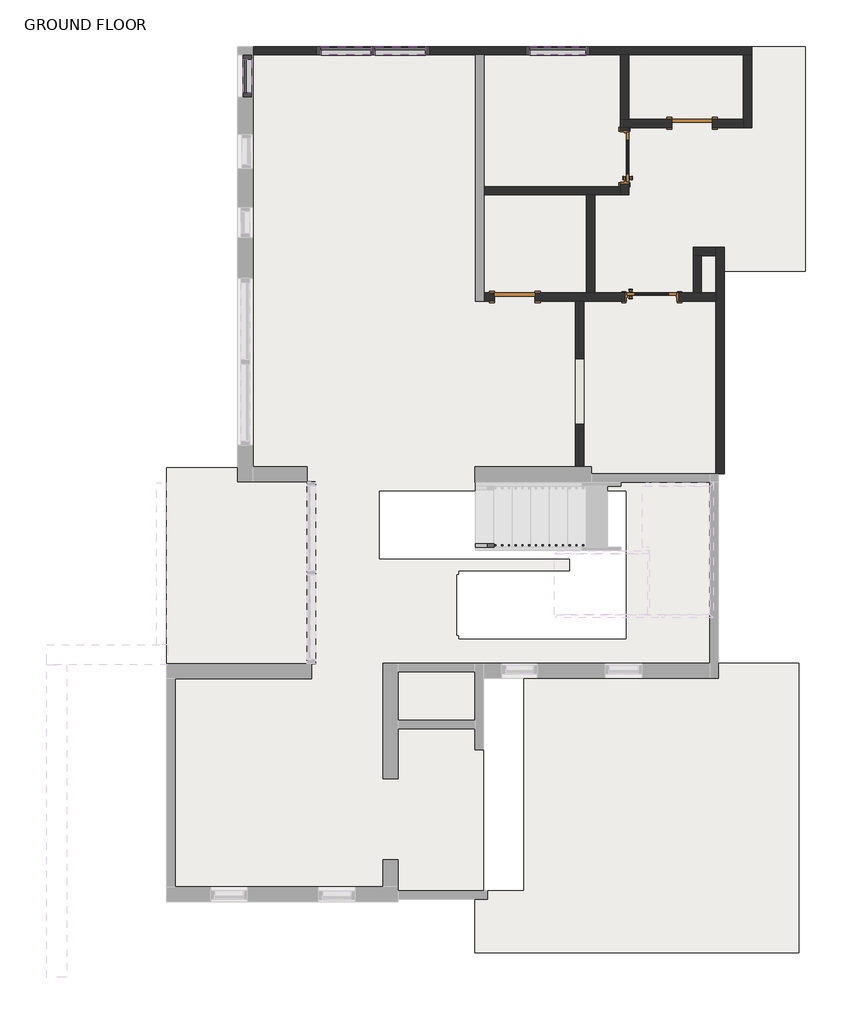
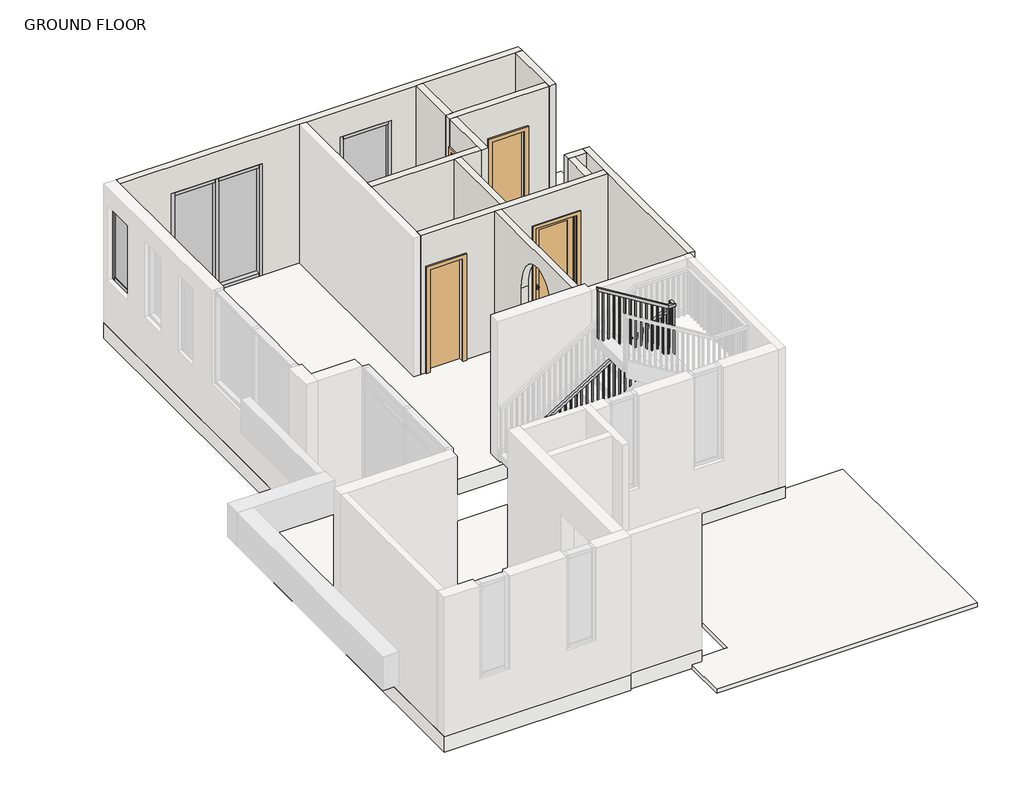
# One storey, part 2 of 3: 15 members, 12 walls, 4 doors, 4 plates, 2 slabs, 1 railing.
"""IFC4 building model written with IfcOpenShell, lengths in millimetres."""

from ifc_helpers import new_model, si_unit, point, frame, origin, origin_with_axes, place, context, project, spatial, polyline, ellipse_curve, trimmed, outline, extrude, faceted_brep, transform, mapped, element, save
from ifc_brep_helpers import plane_surface, extruded_surface, advanced_brep
from components import door_interior_single_1_panel_wood_door_3_x_7_fe7a9c6b, door_interior_single_1_panel_wood_door_3_x_7_d4f3ff50, single_flush_bathroom_2_x7_025d1c86, single_flush_bathroom_2_x7_ccebbf4d, member_de31af64, member_64030597, member_a3a7b6e3, member_71d3972c, member_e3d2676c, member_091e92f8, member_4e4be739, system_panel_glazed_14783ebf, system_panel_glazed_3c43e7a7, system_panel_glazed_fc786b5a

model = new_model("IFC4")

# Units and contexts
model_context = context("Model", 3, world=origin())
ifc_project = project(units=[si_unit("LENGTHUNIT", "METRE", prefix="MILLI")], contexts=[model_context])

# Site, building, storey
site = spatial("IfcSite", under=ifc_project)
building = spatial("IfcBuilding", under=site)
storey = spatial("IfcBuildingStorey", under=building, Name="GROUND FLOOR", Elevation=304.8)

# Doors
placement = place(None, origin())
door_interior_single_1_panel_wood_door_3_x_7_shape = door_interior_single_1_panel_wood_door_3_x_7_fe7a9c6b(model_context)
element("IfcDoor", 1, ObjectType="Door-Interior-Single-1_Panel-Wood : DOOR 3'X 7'", at=placement, inside=storey, context=model_context, shape_type="MappedRepresentation", body=[
    mapped(door_interior_single_1_panel_wood_door_3_x_7_shape, transform((-6017.3265106, -351.9048674, 304.8), x_axis=(0.0, 1.0, 0.0), y_axis=(-1.0, 0.0, 0.0), z_axis=(0.0, 0.0, 1.0))),
])
door_interior_single_1_panel_wood_door_3_x_7_2_shape = door_interior_single_1_panel_wood_door_3_x_7_d4f3ff50(model_context)
element("IfcDoor", 2, ObjectType="Door-Interior-Single-1_Panel-Wood : DOOR 3'X 7'", at=placement, inside=storey, context=model_context, shape_type="MappedRepresentation", body=[
    mapped(door_interior_single_1_panel_wood_door_3_x_7_2_shape, transform((-5610.3998675, -2456.9298674, 304.8), x_axis=(1.0, 0.0, 0.0), y_axis=(0.0, 1.0, 0.0), z_axis=(0.0, 0.0, 1.0))),
])
single_flush_bathroom_2_x7_shape = single_flush_bathroom_2_x7_025d1c86(model_context)
element("IfcDoor", 3, ObjectType="Single-Flush : BATHROOM 2' X7'", at=placement, inside=storey, context=model_context, shape_type="MappedRepresentation", body=[
    mapped(single_flush_bathroom_2_x7_shape, transform((-5004.5015106, 156.0951326, 304.8), x_axis=(1.0, 0.0, 0.0), y_axis=(0.0, 1.0, 0.0), z_axis=(0.0, 0.0, 1.0))),
])
single_flush_bathroom_2_x7_2_shape = single_flush_bathroom_2_x7_ccebbf4d(model_context)
element("IfcDoor", 4, ObjectType="Single-Flush : BATHROOM 2' X7'", at=placement, inside=storey, context=model_context, shape_type="MappedRepresentation", body=[
    mapped(single_flush_bathroom_2_x7_2_shape, transform((-7672.6911408, -2460.1048674, 304.8), x_axis=(-1.0, 0.0, 0.0), y_axis=(0.0, -1.0, 0.0), z_axis=(0.0, 0.0, 1.0))),
])

# Members
member_shape = member_de31af64(model_context)
element("IfcMember", 5, ObjectType="Rectangular Mullion : 2.5\" x 5\" rectangular", at=placement, inside=storey, context=model_context, shape_type="MappedRepresentation", body=[
    mapped(member_shape, transform((-11701.1434938, 1121.2951326, 2682.3285226), x_axis=(0.0, 0.0, 1.0), y_axis=(1.0, 0.0, 0.0), z_axis=(0.0, 1.0, 0.0))),
])
element("IfcMember", 6, ObjectType="Rectangular Mullion : 2.5\" x 5\" rectangular", at=placement, inside=storey, context=model_context, shape_type="MappedRepresentation", body=[
    mapped(member_shape, transform((-11701.1434938, 614.3802108, 1219.2), x_axis=(0.0, 0.0, -1.0), y_axis=(1.0, 0.0, 0.0), z_axis=(0.0, -1.0, 0.0))),
])
member_2_shape = member_64030597(model_context)
element("IfcMember", 7, ObjectType="Rectangular Mullion : 2.5\" x 5\" rectangular", at=placement, inside=storey, context=model_context, shape_type="MappedRepresentation", body=[
    mapped(member_2_shape, transform((-11701.1434938, 1184.7951326, 1219.2), x_axis=(0.0, 1.0, 0.0), y_axis=(1.0, 0.0, 0.0), z_axis=(0.0, 0.0, -1.0))),
])
element("IfcMember", 8, ObjectType="Rectangular Mullion : 2.5\" x 5\" rectangular", at=placement, inside=storey, context=model_context, shape_type="MappedRepresentation", body=[
    mapped(member_2_shape, transform((-11701.1434938, 550.8802108, 2682.3285226), x_axis=(0.0, -1.0, 0.0), y_axis=(1.0, 0.0, 0.0), z_axis=(0.0, 0.0, 1.0))),
])
member_3_shape = member_a3a7b6e3(model_context)
element("IfcMember", 9, ObjectType="Rectangular Mullion : 2.5\" x 5\" rectangular", at=placement, inside=storey, context=model_context, shape_type="MappedRepresentation", body=[
    mapped(member_3_shape, transform((-9021.4434938, 1248.2951326, 2512.8093941), x_axis=(0.0, 0.0, 1.0), y_axis=(0.0, -1.0, 0.0), z_axis=(1.0, 0.0, 0.0))),
])
element("IfcMember", 10, ObjectType="Rectangular Mullion : 2.5\" x 5\" rectangular", at=placement, inside=storey, context=model_context, shape_type="MappedRepresentation", body=[
    mapped(member_3_shape, transform((-9840.5934938, 1248.2951326, 2512.8093941), x_axis=(0.0, 0.0, 1.0), y_axis=(0.0, -1.0, 0.0), z_axis=(1.0, 0.0, 0.0))),
])
element("IfcMember", 11, ObjectType="Rectangular Mullion : 2.5\" x 5\" rectangular", at=placement, inside=storey, context=model_context, shape_type="MappedRepresentation", body=[
    mapped(member_3_shape, transform((-10596.2434938, 1248.2951326, 304.8), x_axis=(0.0, 0.0, -1.0), y_axis=(0.0, -1.0, 0.0), z_axis=(-1.0, 0.0, 0.0))),
])
element("IfcMember", 12, ObjectType="Rectangular Mullion : 2.5\" x 5\" rectangular", at=placement, inside=storey, context=model_context, shape_type="MappedRepresentation", body=[
    mapped(member_3_shape, transform((-9777.0934938, 1248.2951326, 304.8), x_axis=(0.0, 0.0, -1.0), y_axis=(0.0, -1.0, 0.0), z_axis=(-1.0, 0.0, 0.0))),
])
member_4_shape = member_71d3972c(model_context)
element("IfcMember", 13, ObjectType="Rectangular Mullion : 2.5\" x 5\" rectangular", at=placement, inside=storey, context=model_context, shape_type="MappedRepresentation", body=[
    mapped(member_4_shape, transform((-9808.8434938, 1248.2951326, 304.8), x_axis=(1.0, 0.0, 0.0), y_axis=(0.0, -1.0, 0.0), z_axis=(0.0, 0.0, -1.0))),
])
member_5_shape = member_e3d2676c(model_context)
element("IfcMember", 14, ObjectType="Rectangular Mullion : 2.5\" x 5\" rectangular", at=placement, inside=storey, context=model_context, shape_type="MappedRepresentation", body=[
    mapped(member_5_shape, transform((-8957.9434938, 1248.2951326, 304.8), x_axis=(1.0, 0.0, 0.0), y_axis=(0.0, -1.0, 0.0), z_axis=(0.0, 0.0, -1.0))),
])
element("IfcMember", 15, ObjectType="Rectangular Mullion : 2.5\" x 5\" rectangular", at=placement, inside=storey, context=model_context, shape_type="MappedRepresentation", body=[
    mapped(member_5_shape, transform((-10659.7434938, 1248.2951326, 2512.8093941), x_axis=(-1.0, 0.0, 0.0), y_axis=(0.0, -1.0, 0.0), z_axis=(0.0, 0.0, 1.0))),
])
member_6_shape = member_091e92f8(model_context)
element("IfcMember", 16, ObjectType="Rectangular Mullion : 2.5\" x 5\" rectangular", at=placement, inside=storey, context=model_context, shape_type="MappedRepresentation", body=[
    mapped(member_6_shape, transform((-6603.3899211, 1248.2951326, 2525.2042846), x_axis=(0.0, 0.0, 1.0), y_axis=(0.0, -1.0, 0.0), z_axis=(1.0, 0.0, 0.0))),
])
element("IfcMember", 17, ObjectType="Rectangular Mullion : 2.5\" x 5\" rectangular", at=placement, inside=storey, context=model_context, shape_type="MappedRepresentation", body=[
    mapped(member_6_shape, transform((-7447.9399211, 1248.2951326, 304.8), x_axis=(0.0, 0.0, -1.0), y_axis=(0.0, -1.0, 0.0), z_axis=(-1.0, 0.0, 0.0))),
])
member_7_shape = member_4e4be739(model_context)
element("IfcMember", 18, ObjectType="Rectangular Mullion : 2.5\" x 5\" rectangular", at=placement, inside=storey, context=model_context, shape_type="MappedRepresentation", body=[
    mapped(member_7_shape, transform((-6539.8899211, 1248.2951326, 304.8), x_axis=(1.0, 0.0, 0.0), y_axis=(0.0, -1.0, 0.0), z_axis=(0.0, 0.0, -1.0))),
])
element("IfcMember", 19, ObjectType="Rectangular Mullion : 2.5\" x 5\" rectangular", at=placement, inside=storey, context=model_context, shape_type="MappedRepresentation", body=[
    mapped(member_7_shape, transform((-7511.4399211, 1248.2951326, 2525.2042846), x_axis=(-1.0, 0.0, 0.0), y_axis=(0.0, -1.0, 0.0), z_axis=(0.0, 0.0, 1.0))),
])

# Plates
system_panel_glazed_shape = system_panel_glazed_14783ebf(model_context)
element("IfcPlate", 20, ObjectType="System Panel : Glazed", at=placement, inside=storey, context=model_context, shape_type="MappedRepresentation", body=[
    mapped(system_panel_glazed_shape, transform((-11701.1434938, 867.8376717, 1282.7), x_axis=(0.0, 1.0, 0.0), y_axis=(-1.0, 0.0, 0.0), z_axis=(0.0, 0.0, 1.0))),
])
system_panel_glazed_2_shape = system_panel_glazed_3c43e7a7(model_context)
element("IfcPlate", 21, ObjectType="System Panel : Glazed", at=placement, inside=storey, context=model_context, shape_type="MappedRepresentation", body=[
    mapped(system_panel_glazed_2_shape, transform((-10218.4184938, 1248.2951326, 368.3), x_axis=(1.0, 0.0, 0.0), y_axis=(0.0, 1.0, 0.0), z_axis=(0.0, 0.0, 1.0))),
])
element("IfcPlate", 22, ObjectType="System Panel : Glazed", at=placement, inside=storey, context=model_context, shape_type="MappedRepresentation", body=[
    mapped(system_panel_glazed_2_shape, transform((-9399.2684938, 1248.2951326, 368.3), x_axis=(1.0, 0.0, 0.0), y_axis=(0.0, 1.0, 0.0), z_axis=(0.0, 0.0, 1.0))),
])
system_panel_glazed_3_shape = system_panel_glazed_fc786b5a(model_context)
element("IfcPlate", 23, ObjectType="System Panel : Glazed", at=placement, inside=storey, context=model_context, shape_type="MappedRepresentation", body=[
    mapped(system_panel_glazed_3_shape, transform((-7025.6649211, 1248.2951326, 368.3), x_axis=(1.0, 0.0, 0.0), y_axis=(0.0, 1.0, 0.0), z_axis=(0.0, 0.0, 1.0))),
])

# Railing
element("IfcRailing", 24, ObjectType="Handrail - Rectangular", at=placement, inside=storey, context=model_context, shape_type="SolidModel", body=[
    faceted_brep([(-8269.5911408, -6173.9337491, 1390.65), (-8269.5911408, -6173.9337491, 1331.0481634), (-8269.5911408, -6224.7337491, 1331.0481634), (-8269.5911408, -6224.7337491, 1390.65), (-5754.9911408, -6173.9337491, 2933.7), (-5740.6474071, -6173.9337491, 2882.9), (-5740.6474071, -6224.7337491, 2882.9), (-5754.9911408, -6224.7337491, 2933.7), (-5596.7260609, -6173.9337491, 2933.7), (-5596.7260609, -6173.9337491, 2882.9), (-5647.5260609, -6224.7337491, 2882.9), (-5647.5260609, -6224.7337491, 2933.7), (-5596.7260609, -6251.7310793, 2933.7), (-5596.7260609, -6302.5310793, 2882.9), (-5647.5260609, -6302.5310793, 2882.9), (-5647.5260609, -6251.7310793, 2933.7), (-5596.7260609, -6251.7310793, 3151.9090909), (-5596.7260609, -6302.5310793, 3101.1090909), (-5647.5260609, -6302.5310793, 3101.1090909), (-5647.5260609, -6251.7310793, 3151.9090909), (-5596.7260609, -6378.7310793, 3151.9090909), (-5596.7260609, -6378.7310793, 3101.1090909), (-5647.5260609, -6327.9310793, 3101.1090909), (-5647.5260609, -6327.9310793, 3151.9090909), (-5723.7260609, -6378.7310793, 3151.9090909), (-5738.0697946, -6378.7310793, 3101.1090909), (-5738.0697946, -6327.9310793, 3101.1090909), (-5723.7260609, -6327.9310793, 3151.9090909), (-7044.5260609, -6378.7310793, 3962.4), (-7044.5260609, -6327.9310793, 3962.4), (-7044.5260609, -6327.9310793, 3902.7981634), (-7044.5260609, -6378.7310793, 3902.7981634)], [[[0, 1, 2, 3]], [[1, 0, 4, 5]], [[2, 1, 5, 6]], [[3, 2, 6, 7]], [[0, 3, 7, 4]], [[5, 4, 8, 9]], [[6, 5, 9, 10]], [[7, 6, 10, 11]], [[4, 7, 11, 8]], [[9, 8, 12, 13]], [[10, 9, 13, 14]], [[11, 10, 14, 15]], [[8, 11, 15, 12]], [[13, 12, 16, 17]], [[14, 13, 17, 18]], [[15, 14, 18, 19]], [[12, 15, 19, 16]], [[17, 16, 20, 21]], [[18, 17, 21, 22]], [[19, 18, 22, 23]], [[16, 19, 23, 20]], [[21, 20, 24, 25]], [[22, 21, 25, 26]], [[23, 22, 26, 27]], [[20, 23, 27, 24]], [[28, 29, 30, 31]], [[25, 24, 28, 31]], [[26, 25, 31, 30]], [[27, 26, 30, 29]], [[24, 27, 29, 28]]]),
    extrude(outline(polyline([(3834.6078225, -6933.4010609), (3846.2975952, -6952.4510609), (2876.55, -6952.4510609), (2876.55, -6933.4010609), (3834.6078225, -6933.4010609)])), frame((0.0, -6362.8560793, 0.0), z_axis=(0.0, 1.0, 0.0), x_axis=(0.0, 0.0, 1.0)), (0.0, 0.0, 1.0), 19.05),
    extrude(outline(polyline([(3772.2623679, -6831.8010609), (3783.9521407, -6850.8510609), (2876.55, -6850.8510609), (2876.55, -6831.8010609), (3772.2623679, -6831.8010609)])), frame((0.0, -6362.8560793, 0.0), z_axis=(0.0, 1.0, 0.0), x_axis=(0.0, 0.0, 1.0)), (0.0, 0.0, 1.0), 19.05),
    extrude(outline(polyline([(3709.9169134, -6730.2010609), (3721.6066861, -6749.2510609), (2705.1, -6749.2510609), (2705.1, -6730.2010609), (3709.9169134, -6730.2010609)])), frame((0.0, -6362.8560793, 0.0), z_axis=(0.0, 1.0, 0.0), x_axis=(0.0, 0.0, 1.0)), (0.0, 0.0, 1.0), 19.05),
    extrude(outline(polyline([(3647.5714589, -6628.6010609), (3659.2612316, -6647.6510609), (2705.1, -6647.6510609), (2705.1, -6628.6010609), (3647.5714589, -6628.6010609)])), frame((0.0, -6362.8560793, 0.0), z_axis=(0.0, 1.0, 0.0), x_axis=(0.0, 0.0, 1.0)), (0.0, 0.0, 1.0), 19.05),
    extrude(outline(polyline([(3585.2260043, -6527.0010609), (3596.915777, -6546.0510609), (2705.1, -6546.0510609), (2705.1, -6527.0010609), (3585.2260043, -6527.0010609)])), frame((0.0, -6362.8560793, 0.0), z_axis=(0.0, 1.0, 0.0), x_axis=(0.0, 0.0, 1.0)), (0.0, 0.0, 1.0), 19.05),
    extrude(outline(polyline([(3522.8805498, -6425.4010609), (3534.5703225, -6444.4510609), (2533.65, -6444.4510609), (2533.65, -6425.4010609), (3522.8805498, -6425.4010609)])), frame((0.0, -6362.8560793, 0.0), z_axis=(0.0, 1.0, 0.0), x_axis=(0.0, 0.0, 1.0)), (0.0, 0.0, 1.0), 19.05),
    extrude(outline(polyline([(3460.5350952, -6323.8010609), (3472.2248679, -6342.8510609), (2533.65, -6342.8510609), (2533.65, -6323.8010609), (3460.5350952, -6323.8010609)])), frame((0.0, -6362.8560793, 0.0), z_axis=(0.0, 1.0, 0.0), x_axis=(0.0, 0.0, 1.0)), (0.0, 0.0, 1.0), 19.05),
    extrude(outline(polyline([(3398.1896407, -6222.2010609), (3409.8794134, -6241.2510609), (2533.65, -6241.2510609), (2533.65, -6222.2010609), (3398.1896407, -6222.2010609)])), frame((0.0, -6362.8560793, 0.0), z_axis=(0.0, 1.0, 0.0), x_axis=(0.0, 0.0, 1.0)), (0.0, 0.0, 1.0), 19.05),
    extrude(outline(polyline([(3335.8441861, -6120.6010609), (3347.5339589, -6139.6510609), (2362.2, -6139.6510609), (2362.2, -6120.6010609), (3335.8441861, -6120.6010609)])), frame((0.0, -6362.8560793, 0.0), z_axis=(0.0, 1.0, 0.0), x_axis=(0.0, 0.0, 1.0)), (0.0, 0.0, 1.0), 19.05),
    extrude(outline(polyline([(3273.4987316, -6019.0010609), (3285.1885043, -6038.0510609), (2362.2, -6038.0510609), (2362.2, -6019.0010609), (3273.4987316, -6019.0010609)])), frame((0.0, -6362.8560793, 0.0), z_axis=(0.0, 1.0, 0.0), x_axis=(0.0, 0.0, 1.0)), (0.0, 0.0, 1.0), 19.05),
    extrude(outline(polyline([(3211.153277, -5917.4010609), (3222.8430498, -5936.4510609), (2362.2, -5936.4510609), (2362.2, -5917.4010609), (3211.153277, -5917.4010609)])), frame((0.0, -6362.8560793, 0.0), z_axis=(0.0, 1.0, 0.0), x_axis=(0.0, 0.0, 1.0)), (0.0, 0.0, 1.0), 19.05),
    extrude(outline(polyline([(3148.8078225, -5815.8010609), (3160.4975952, -5834.8510609), (2190.75, -5834.8510609), (2190.75, -5815.8010609), (3148.8078225, -5815.8010609)])), frame((0.0, -6362.8560793, 0.0), z_axis=(0.0, 1.0, 0.0), x_axis=(0.0, 0.0, 1.0)), (0.0, 0.0, 1.0), 19.05),
    extrude(outline(polyline([(3086.4623679, -5714.2010609), (3098.1521407, -5733.2510609), (2190.75, -5733.2510609), (2190.75, -5714.2010609), (3086.4623679, -5714.2010609)])), frame((0.0, -6362.8560793, 0.0), z_axis=(0.0, 1.0, 0.0), x_axis=(0.0, 0.0, 1.0)), (0.0, 0.0, 1.0), 19.05),
    extrude(outline(polyline([(-5631.6510609, -6291.4087491), (-5612.6010609, -6291.4087491), (-5612.6010609, -6310.4587491), (-5631.6510609, -6310.4587491), (-5631.6510609, -6291.4087491)])), frame((0.0, 0.0, 2019.3), z_axis=(0.0, 0.0, 1.0), x_axis=(1.0, 0.0, 0.0)), (0.0, 0.0, 1.0), 1081.8090909),
    extrude(outline(polyline([(-5662.9161408, -6208.8587491), (-5662.9161408, -6189.8087491), (-5643.8661408, -6189.8087491), (-5643.8661408, -6208.8587491), (-5662.9161408, -6208.8587491)])), frame((0.0, 0.0, 2019.3), z_axis=(0.0, 0.0, 1.0), x_axis=(1.0, 0.0, 0.0)), (0.0, 0.0, 1.0), 863.6),
    extrude(outline(polyline([(2833.1839589, -5821.6661408), (2821.4941861, -5840.7161408), (1847.85, -5840.7161408), (1847.85, -5821.6661408), (2833.1839589, -5821.6661408)])), frame((0.0, -6208.8587491, 0.0), z_axis=(0.0, 1.0, 0.0), x_axis=(0.0, 0.0, 1.0)), (0.0, 0.0, 1.0), 19.05),
    extrude(outline(polyline([(2770.8385043, -5923.2661408), (2759.1487316, -5942.3161408), (1847.85, -5942.3161408), (1847.85, -5923.2661408), (2770.8385043, -5923.2661408)])), frame((0.0, -6208.8587491, 0.0), z_axis=(0.0, 1.0, 0.0), x_axis=(0.0, 0.0, 1.0)), (0.0, 0.0, 1.0), 19.05),
    extrude(outline(polyline([(2708.4930498, -6024.8661408), (2696.803277, -6043.9161408), (1847.85, -6043.9161408), (1847.85, -6024.8661408), (2708.4930498, -6024.8661408)])), frame((0.0, -6208.8587491, 0.0), z_axis=(0.0, 1.0, 0.0), x_axis=(0.0, 0.0, 1.0)), (0.0, 0.0, 1.0), 19.05),
    extrude(outline(polyline([(2646.1475952, -6126.4661408), (2634.4578225, -6145.5161408), (1676.4, -6145.5161408), (1676.4, -6126.4661408), (2646.1475952, -6126.4661408)])), frame((0.0, -6208.8587491, 0.0), z_axis=(0.0, 1.0, 0.0), x_axis=(0.0, 0.0, 1.0)), (0.0, 0.0, 1.0), 19.05),
    extrude(outline(polyline([(2583.8021407, -6228.0661408), (2572.1123679, -6247.1161408), (1676.4, -6247.1161408), (1676.4, -6228.0661408), (2583.8021407, -6228.0661408)])), frame((0.0, -6208.8587491, 0.0), z_axis=(0.0, 1.0, 0.0), x_axis=(0.0, 0.0, 1.0)), (0.0, 0.0, 1.0), 19.05),
    extrude(outline(polyline([(2521.4566861, -6329.6661408), (2509.7669134, -6348.7161408), (1504.95, -6348.7161408), (1504.95, -6329.6661408), (2521.4566861, -6329.6661408)])), frame((0.0, -6208.8587491, 0.0), z_axis=(0.0, 1.0, 0.0), x_axis=(0.0, 0.0, 1.0)), (0.0, 0.0, 1.0), 19.05),
    extrude(outline(polyline([(2459.1112316, -6431.2661408), (2447.4214589, -6450.3161408), (1504.95, -6450.3161408), (1504.95, -6431.2661408), (2459.1112316, -6431.2661408)])), frame((0.0, -6208.8587491, 0.0), z_axis=(0.0, 1.0, 0.0), x_axis=(0.0, 0.0, 1.0)), (0.0, 0.0, 1.0), 19.05),
    extrude(outline(polyline([(2396.765777, -6532.8661408), (2385.0760043, -6551.9161408), (1504.95, -6551.9161408), (1504.95, -6532.8661408), (2396.765777, -6532.8661408)])), frame((0.0, -6208.8587491, 0.0), z_axis=(0.0, 1.0, 0.0), x_axis=(0.0, 0.0, 1.0)), (0.0, 0.0, 1.0), 19.05),
    extrude(outline(polyline([(2334.4203225, -6634.4661408), (2322.7305498, -6653.5161408), (1333.5, -6653.5161408), (1333.5, -6634.4661408), (2334.4203225, -6634.4661408)])), frame((0.0, -6208.8587491, 0.0), z_axis=(0.0, 1.0, 0.0), x_axis=(0.0, 0.0, 1.0)), (0.0, 0.0, 1.0), 19.05),
    extrude(outline(polyline([(2272.0748679, -6736.0661408), (2260.3850952, -6755.1161408), (1333.5, -6755.1161408), (1333.5, -6736.0661408), (2272.0748679, -6736.0661408)])), frame((0.0, -6208.8587491, 0.0), z_axis=(0.0, 1.0, 0.0), x_axis=(0.0, 0.0, 1.0)), (0.0, 0.0, 1.0), 19.05),
    extrude(outline(polyline([(2209.7294134, -6837.6661408), (2198.0396407, -6856.7161408), (1333.5, -6856.7161408), (1333.5, -6837.6661408), (2209.7294134, -6837.6661408)])), frame((0.0, -6208.8587491, 0.0), z_axis=(0.0, 1.0, 0.0), x_axis=(0.0, 0.0, 1.0)), (0.0, 0.0, 1.0), 19.05),
    extrude(outline(polyline([(2147.3839589, -6939.2661408), (2135.6941861, -6958.3161408), (1162.05, -6958.3161408), (1162.05, -6939.2661408), (2147.3839589, -6939.2661408)])), frame((0.0, -6208.8587491, 0.0), z_axis=(0.0, 1.0, 0.0), x_axis=(0.0, 0.0, 1.0)), (0.0, 0.0, 1.0), 19.05),
    extrude(outline(polyline([(2085.0385043, -7040.8661408), (2073.3487316, -7059.9161408), (1162.05, -7059.9161408), (1162.05, -7040.8661408), (2085.0385043, -7040.8661408)])), frame((0.0, -6208.8587491, 0.0), z_axis=(0.0, 1.0, 0.0), x_axis=(0.0, 0.0, 1.0)), (0.0, 0.0, 1.0), 19.05),
    extrude(outline(polyline([(2022.6930498, -7142.4661408), (2011.003277, -7161.5161408), (1162.05, -7161.5161408), (1162.05, -7142.4661408), (2022.6930498, -7142.4661408)])), frame((0.0, -6208.8587491, 0.0), z_axis=(0.0, 1.0, 0.0), x_axis=(0.0, 0.0, 1.0)), (0.0, 0.0, 1.0), 19.05),
    extrude(outline(polyline([(1960.3475952, -7244.0661408), (1948.6578225, -7263.1161408), (990.6, -7263.1161408), (990.6, -7244.0661408), (1960.3475952, -7244.0661408)])), frame((0.0, -6208.8587491, 0.0), z_axis=(0.0, 1.0, 0.0), x_axis=(0.0, 0.0, 1.0)), (0.0, 0.0, 1.0), 19.05),
    extrude(outline(polyline([(1898.0021407, -7345.6661408), (1886.3123679, -7364.7161408), (990.6, -7364.7161408), (990.6, -7345.6661408), (1898.0021407, -7345.6661408)])), frame((0.0, -6208.8587491, 0.0), z_axis=(0.0, 1.0, 0.0), x_axis=(0.0, 0.0, 1.0)), (0.0, 0.0, 1.0), 19.05),
    extrude(outline(polyline([(1835.6566861, -7447.2661408), (1823.9669134, -7466.3161408), (819.15, -7466.3161408), (819.15, -7447.2661408), (1835.6566861, -7447.2661408)])), frame((0.0, -6208.8587491, 0.0), z_axis=(0.0, 1.0, 0.0), x_axis=(0.0, 0.0, 1.0)), (0.0, 0.0, 1.0), 19.05),
    extrude(outline(polyline([(1773.3112316, -7548.8661408), (1761.6214589, -7567.9161408), (819.15, -7567.9161408), (819.15, -7548.8661408), (1773.3112316, -7548.8661408)])), frame((0.0, -6208.8587491, 0.0), z_axis=(0.0, 1.0, 0.0), x_axis=(0.0, 0.0, 1.0)), (0.0, 0.0, 1.0), 19.05),
    extrude(outline(polyline([(1710.965777, -7650.4661408), (1699.2760043, -7669.5161408), (819.15, -7669.5161408), (819.15, -7650.4661408), (1710.965777, -7650.4661408)])), frame((0.0, -6208.8587491, 0.0), z_axis=(0.0, 1.0, 0.0), x_axis=(0.0, 0.0, 1.0)), (0.0, 0.0, 1.0), 19.05),
    extrude(outline(polyline([(1648.6203225, -7752.0661408), (1636.9305498, -7771.1161408), (647.7, -7771.1161408), (647.7, -7752.0661408), (1648.6203225, -7752.0661408)])), frame((0.0, -6208.8587491, 0.0), z_axis=(0.0, 1.0, 0.0), x_axis=(0.0, 0.0, 1.0)), (0.0, 0.0, 1.0), 19.05),
    extrude(outline(polyline([(1586.2748679, -7853.6661408), (1574.5850952, -7872.7161408), (647.7, -7872.7161408), (647.7, -7853.6661408), (1586.2748679, -7853.6661408)])), frame((0.0, -6208.8587491, 0.0), z_axis=(0.0, 1.0, 0.0), x_axis=(0.0, 0.0, 1.0)), (0.0, 0.0, 1.0), 19.05),
    extrude(outline(polyline([(1523.9294134, -7955.2661408), (1512.2396407, -7974.3161408), (647.7, -7974.3161408), (647.7, -7955.2661408), (1523.9294134, -7955.2661408)])), frame((0.0, -6208.8587491, 0.0), z_axis=(0.0, 1.0, 0.0), x_axis=(0.0, 0.0, 1.0)), (0.0, 0.0, 1.0), 19.05),
    extrude(outline(polyline([(1461.5839589, -8056.8661408), (1449.8941861, -8075.9161408), (476.25, -8075.9161408), (476.25, -8056.8661408), (1461.5839589, -8056.8661408)])), frame((0.0, -6208.8587491, 0.0), z_axis=(0.0, 1.0, 0.0), x_axis=(0.0, 0.0, 1.0)), (0.0, 0.0, 1.0), 19.05),
    extrude(outline(polyline([(1399.2385043, -8158.4661408), (1387.5487316, -8177.5161408), (476.25, -8177.5161408), (476.25, -8158.4661408), (1399.2385043, -8158.4661408)])), frame((0.0, -6208.8587491, 0.0), z_axis=(0.0, 1.0, 0.0), x_axis=(0.0, 0.0, 1.0)), (0.0, 0.0, 1.0), 19.05),
    extrude(outline(polyline([(-5631.6510609, -6343.8060793), (-5612.6010609, -6343.8060793), (-5612.6010609, -6362.8560793), (-5631.6510609, -6362.8560793), (-5631.6510609, -6343.8060793)])), frame((0.0, 0.0, 2019.3), z_axis=(0.0, 0.0, 1.0), x_axis=(1.0, 0.0, 0.0)), (0.0, 0.0, 1.0), 1081.8090909),
    extrude(outline(polyline([(-5631.6510609, -6208.8587491), (-5631.6510609, -6189.8087491), (-5612.6010609, -6189.8087491), (-5612.6010609, -6208.8587491), (-5631.6510609, -6208.8587491)])), frame((0.0, 0.0, 2019.3), z_axis=(0.0, 0.0, 1.0), x_axis=(1.0, 0.0, 0.0)), (0.0, 0.0, 1.0), 863.6),
    extrude(outline(polyline([(2879.9430498, -5745.4661408), (2868.253277, -5764.5161408), (2019.3, -5764.5161408), (2019.3, -5745.4661408), (2879.9430498, -5745.4661408)])), frame((0.0, -6208.8587491, 0.0), z_axis=(0.0, 1.0, 0.0), x_axis=(0.0, 0.0, 1.0)), (0.0, 0.0, 1.0), 19.05),
    extrude(outline(polyline([(3891.1083907, -7025.4760609), (3902.7981634, -7044.5260609), (2876.55, -7044.5260609), (2876.55, -7025.4760609), (3891.1083907, -7025.4760609)])), frame((0.0, -6362.8560793, 0.0), z_axis=(0.0, 1.0, 0.0), x_axis=(0.0, 0.0, 1.0)), (0.0, 0.0, 1.0), 19.05),
    extrude(outline(polyline([(1342.7379361, -8250.5411408), (1331.0481634, -8269.5911408), (476.25, -8269.5911408), (476.25, -8250.5411408), (1342.7379361, -8250.5411408)])), frame((0.0, -6208.8587491, 0.0), z_axis=(0.0, 1.0, 0.0), x_axis=(0.0, 0.0, 1.0)), (0.0, 0.0, 1.0), 19.05),
])

# Slabs
element("IfcSlab", 25, ObjectType="MARBLE FLOORING 1'", at=placement, inside=storey, context=model_context, shape_type="SweptSolid", body=[
    extrude(outline(polyline([(-8087.622653, -11530.1453012), (-9433.822653, -11530.1453012), (-9433.822653, -11568.2453012), (-12920.5906521, -11568.2453012), (-12920.5906521, -5027.4864969), (-11849.8015106, -5027.4864969), (-11849.8015106, 1311.7951326), (-3297.4727979, 1311.7951326), (-3297.4727979, -2071.8337491), (-4516.6727979, -2071.8337491), (-4516.6727979, -5119.8337491), (-4605.5727979, -5119.8337491), (-4605.5727979, -8203.7830995), (-8147.3960918, -8203.7830995), (-8147.3960918, -11403.1453012), (-8087.622653, -11403.1453012), (-8087.622653, -11530.1453012)]), holes=[polyline([(-8549.4760609, -7553.4810793), (-8517.7260609, -7553.4810793), (-8517.7260609, -7604.2810793), (-6003.1260609, -7604.2810793), (-6003.1260609, -5382.5504041), (-9709.3703437, -5382.5504041), (-9709.3703437, -6398.5504041), (-6841.3260609, -6398.5504041), (-6841.3260609, -6588.2810793), (-8517.7260609, -6588.2810793), (-8517.7260609, -6639.0810793), (-8549.4760609, -6639.0810793), (-8549.4760609, -7553.4810793)])]), origin_with_axes(), (0.0, 0.0, 1.0), 304.8),
])
element("IfcSlab", 26, ObjectType="VERANDA FLOORING 3\"", at=placement, inside=storey, context=model_context, shape_type="SweptSolid", body=[
    extrude(outline(polyline([(-3395.0260735, -7975.1830995), (-3395.0260735, -12330.4921987), (-8271.8260735, -12330.4921987), (-8271.8260735, -11530.1453012), (-8087.622653, -11530.1453012), (-8087.622653, -11403.1453012), (-7537.7960918, -11403.1453012), (-7537.7960918, -8203.7830995), (-4605.5727979, -8203.7830995), (-4605.5727979, -7975.1830995), (-3395.0260735, -7975.1830995)])), origin_with_axes(), (0.0, 0.0, 1.0), 76.2),
])

# Walls
element("IfcWall", 27, ObjectType="INTERIOR WALL PAINT 5\"", at=placement, inside=storey, context=model_context, shape_type="Brep", body=[
    faceted_brep([(-4102.8015106, 1184.7951326, 3048.0), (-4229.8015106, 1184.7951326, 3048.0), (-5957.0015106, 1184.7951326, 3048.0), (-6084.0015106, 1184.7951326, 3048.0), (-8142.5911408, 1184.7951326, 3048.0), (-8269.5911408, 1184.7951326, 3048.0), (-11621.2015106, 1184.7951326, 3048.0), (-11621.2015106, 1184.7951326, 2682.3285226), (-11621.2015106, 1184.7951326, 1219.2), (-11621.2015106, 1184.7951326, 304.8), (-10659.7434938, 1184.7951326, 304.8), (-10659.7434938, 1184.7951326, 2512.8093941), (-8957.9434938, 1184.7951326, 2512.8093941), (-8957.9434938, 1184.7951326, 304.8), (-8269.5911408, 1184.7951326, 304.8), (-8142.5911408, 1184.7951326, 304.8), (-7511.4399211, 1184.7951326, 304.8), (-7511.4399211, 1184.7951326, 2525.2042846), (-6539.8899211, 1184.7951326, 2525.2042846), (-6539.8899211, 1184.7951326, 304.8), (-6084.0015106, 1184.7951326, 304.8), (-5957.0015106, 1184.7951326, 304.8), (-4229.8015106, 1184.7951326, 304.8), (-4102.8015106, 1184.7951326, 304.8), (-11621.2015106, 1311.7951326, 3048.0), (-4102.8015106, 1311.7951326, 3048.0), (-4102.8015106, 1311.7951326, 304.8), (-6539.8899211, 1311.7951326, 304.8), (-6539.8899211, 1311.7951326, 2525.2042846), (-7511.4399211, 1311.7951326, 2525.2042846), (-7511.4399211, 1311.7951326, 304.8), (-8957.9434938, 1311.7951326, 304.8), (-8957.9434938, 1311.7951326, 2512.8093941), (-10659.7434938, 1311.7951326, 2512.8093941), (-10659.7434938, 1311.7951326, 304.8), (-11621.2015106, 1311.7951326, 304.8)], [[[0, 1, 2, 3, 4, 5, 6, 7, 8, 9, 10, 11, 12, 13, 14, 15, 16, 17, 18, 19, 20, 21, 22, 23]], [[24, 25, 26, 27, 28, 29, 30, 31, 32, 33, 34, 35]], [[9, 35, 34, 10]], [[26, 23, 22, 21, 20, 19, 27]], [[13, 31, 30, 16, 15, 14]], [[6, 5, 4, 3, 2, 1, 0, 25, 24]], [[9, 8, 7, 6, 24, 35]], [[0, 23, 26, 25]], [[33, 11, 10, 34]], [[11, 33, 32, 12]], [[12, 32, 31, 13]], [[29, 17, 16, 30]], [[17, 29, 28, 18]], [[18, 28, 27, 19]]]),
])
element("IfcWall", 28, ObjectType="INTERIOR WALL PAINT 5\"", at=placement, inside=storey, context=model_context, shape_type="Brep", body=[
    faceted_brep([(-4229.8015106, 1184.7951326, 304.8), (-4229.8015106, 219.5951326, 304.8), (-4229.8015106, 92.5951326, 304.8), (-4229.8015106, 92.5951326, 3048.0), (-4229.8015106, 219.5951326, 3048.0), (-4229.8015106, 1184.7951326, 3048.0), (-4102.8015106, 1184.7951326, 304.8), (-4102.8015106, 1184.7951326, 3048.0), (-4102.8015106, 92.5951326, 3048.0), (-4102.8015106, 92.5951326, 304.8)], [[[0, 1, 2, 3, 4, 5]], [[6, 7, 8, 9]], [[2, 1, 0, 6, 9]], [[5, 4, 3, 8, 7]], [[0, 5, 7, 6]], [[3, 2, 9, 8]]]),
])
element("IfcWall", 29, ObjectType="INTERIOR WALL PAINT 5\"", at=placement, inside=storey, context=model_context, shape_type="Brep", body=[
    faceted_brep([(-4229.8015106, 219.5951326, 304.8), (-4699.7015106, 219.5951326, 304.8), (-4699.7015106, 219.5951326, 2336.8), (-5309.3015106, 219.5951326, 2336.8), (-5309.3015106, 219.5951326, 304.8), (-5957.0015106, 219.5951326, 304.8), (-6084.0015106, 219.5951326, 304.8), (-6084.0015106, 219.5951326, 3048.0), (-5957.0015106, 219.5951326, 3048.0), (-4229.8015106, 219.5951326, 3048.0), (-4699.7015106, 92.5951326, 2336.8), (-4699.7015106, 92.5951326, 304.8), (-4229.8015106, 92.5951326, 304.8), (-4229.8015106, 92.5951326, 3048.0), (-5957.0015106, 92.5951326, 3048.0), (-6084.0015106, 92.5951326, 3048.0), (-6084.0015106, 92.5951326, 304.8), (-5957.0015106, 92.5951326, 304.8), (-5309.3015106, 92.5951326, 304.8), (-5309.3015106, 92.5951326, 2336.8)], [[[0, 1, 2, 3, 4, 5, 6, 7, 8, 9]], [[10, 11, 12, 13, 14, 15, 16, 17, 18, 19]], [[12, 11, 1, 0]], [[18, 17, 16, 6, 5, 4]], [[9, 8, 7, 15, 14, 13]], [[0, 9, 13, 12]], [[7, 6, 16, 15]], [[2, 1, 11, 10]], [[3, 2, 10, 19]], [[4, 3, 19, 18]]]),
])
element("IfcWall", 30, ObjectType="INTERIOR WALL PAINT 5\"", at=placement, inside=storey, context=model_context, shape_type="SweptSolid", body=[
    extrude(outline(polyline([(-5957.0015106, 1184.7951326), (-5957.0015106, 219.5951326), (-6084.0015106, 219.5951326), (-6084.0015106, 1184.7951326), (-5957.0015106, 1184.7951326)])), frame((0.0, 0.0, 304.8), z_axis=(0.0, 0.0, 1.0), x_axis=(1.0, 0.0, 0.0)), (0.0, 0.0, 1.0), 2743.2),
])
element("IfcWall", 31, ObjectType="INTERIOR WALL PAINT 5\"", at=placement, inside=storey, context=model_context, shape_type="Brep", body=[
    faceted_brep([(-4643.6727979, -2523.6048674, 3048.0), (-6631.2911408, -2523.6048674, 3048.0), (-6758.2911408, -2523.6048674, 3048.0), (-8142.5911408, -2523.6048674, 3048.0), (-8142.5911408, -2523.6048674, 304.8), (-7977.4911408, -2523.6048674, 304.8), (-7977.4911408, -2523.6048674, 2336.8), (-7367.8911408, -2523.6048674, 2336.8), (-7367.8911408, -2523.6048674, 304.8), (-6758.2911408, -2523.6048674, 304.8), (-6631.2911408, -2523.6048674, 304.8), (-6016.7998675, -2523.6048674, 304.8), (-6016.7998675, -2523.6048674, 2463.8), (-5203.9998675, -2523.6048674, 2463.8), (-5203.9998675, -2523.6048674, 304.8), (-4643.6727979, -2523.6048674, 304.8), (-8142.5911408, -2396.6048674, 3048.0), (-6593.1911408, -2396.6048674, 3048.0), (-6466.1911408, -2396.6048674, 3048.0), (-4988.0998675, -2396.6048674, 3048.0), (-4861.0998675, -2396.6048674, 3048.0), (-4643.6727979, -2396.6048674, 3048.0), (-4643.6727979, -2396.6048674, 304.8), (-4861.0998675, -2396.6048674, 304.8), (-4988.0998675, -2396.6048674, 304.8), (-5203.9998675, -2396.6048674, 304.8), (-5203.9998675, -2396.6048674, 2463.8), (-6016.7998675, -2396.6048674, 2463.8), (-6016.7998675, -2396.6048674, 304.8), (-6466.1911408, -2396.6048674, 304.8), (-6593.1911408, -2396.6048674, 304.8), (-7367.8911408, -2396.6048674, 304.8), (-7367.8911408, -2396.6048674, 2336.8), (-7977.4911408, -2396.6048674, 2336.8), (-7977.4911408, -2396.6048674, 304.8), (-8142.5911408, -2396.6048674, 304.8)], [[[0, 1, 2, 3, 4, 5, 6, 7, 8, 9, 10, 11, 12, 13, 14, 15]], [[16, 17, 18, 19, 20, 21, 22, 23, 24, 25, 26, 27, 28, 29, 30, 31, 32, 33, 34, 35]], [[4, 35, 34, 5]], [[22, 15, 14, 25, 24, 23]], [[8, 31, 30, 29, 28, 11, 10, 9]], [[3, 2, 1, 0, 21, 20, 19, 18, 17, 16]], [[4, 3, 16, 35]], [[0, 15, 22, 21]], [[6, 5, 34, 33]], [[7, 6, 33, 32]], [[8, 7, 32, 31]], [[13, 26, 25, 14]], [[26, 13, 12, 27]], [[27, 12, 11, 28]]]),
])
element("IfcWall", 32, ObjectType="INTERIOR WALL PAINT 5\"", at=placement, inside=storey, context=model_context, shape_type="SweptSolid", body=[
    extrude(outline(polyline([(-6466.1911408, -923.4048674), (-6466.1911408, -2396.6048674), (-6593.1911408, -2396.6048674), (-6593.1911408, -923.4048674), (-6466.1911408, -923.4048674)])), frame((0.0, 0.0, 304.8), z_axis=(0.0, 0.0, 1.0), x_axis=(1.0, 0.0, 0.0)), (0.0, 0.0, 1.0), 2743.2),
])
element("IfcWall", 33, ObjectType="INTERIOR WALL PAINT 5\"", at=placement, inside=storey, context=model_context, shape_type="Brep", body=[
    faceted_brep([(-6084.0015106, -923.4048674, 3048.0), (-6084.0015106, -796.4048674, 3048.0), (-6084.0015106, 92.5951326, 3048.0), (-6084.0015106, 92.5951326, 304.8), (-6084.0015106, 54.4951326, 304.8), (-6084.0015106, 54.4951326, 2463.8), (-6084.0015106, -758.3048674, 2463.8), (-6084.0015106, -758.3048674, 304.8), (-6084.0015106, -796.4048674, 304.8), (-6084.0015106, -923.4048674, 304.8), (-5957.0015106, 92.5951326, 3048.0), (-5957.0015106, -923.4048674, 3048.0), (-5957.0015106, -923.4048674, 304.8), (-5957.0015106, -758.3048674, 304.8), (-5957.0015106, -758.3048674, 2463.8), (-5957.0015106, 54.4951326, 2463.8), (-5957.0015106, 54.4951326, 304.8), (-5957.0015106, 92.5951326, 304.8)], [[[0, 1, 2, 3, 4, 5, 6, 7, 8, 9]], [[10, 11, 12, 13, 14, 15, 16, 17]], [[3, 17, 16, 4]], [[12, 9, 8, 7, 13]], [[2, 1, 0, 11, 10]], [[3, 2, 10, 17]], [[0, 9, 12, 11]], [[15, 5, 4, 16]], [[5, 15, 14, 6]], [[6, 14, 13, 7]]]),
])
element("IfcWall", 34, ObjectType="INTERIOR WALL PAINT 5\"", at=placement, inside=storey, context=model_context, shape_type="Brep", body=[
    faceted_brep([(-6084.0015106, -796.4048674, 304.8), (-8142.5911408, -796.4048674, 304.8), (-8142.5911408, -796.4048674, 3048.0), (-6084.0015106, -796.4048674, 3048.0), (-6084.0015106, -923.4048674, 304.8), (-6084.0015106, -923.4048674, 3048.0), (-6466.1911408, -923.4048674, 3048.0), (-6593.1911408, -923.4048674, 3048.0), (-8142.5911408, -923.4048674, 3048.0), (-8142.5911408, -923.4048674, 304.8), (-6593.1911408, -923.4048674, 304.8), (-6466.1911408, -923.4048674, 304.8)], [[[0, 1, 2, 3]], [[4, 5, 6, 7, 8, 9, 10, 11]], [[1, 0, 4, 11, 10, 9]], [[3, 2, 8, 7, 6, 5]], [[0, 3, 5, 4]], [[2, 1, 9, 8]]]),
])
element("IfcWall", 35, ObjectType="INTERIOR WALL PAINT 5\"", at=placement, inside=storey, context=model_context, shape_type="AdvancedBrep", body=[
    advanced_brep(
    [(-6758.2911408, -2523.6048674, 304.8), (-6758.2911408, -5018.2337491, 304.8), (-6758.2911408, -5018.2337491, 3048.0), (-6758.2911408, -2523.6048674, 3048.0), (-6758.2911408, -4372.8519167, 474.3743557), (-6758.2911408, -3388.6019167, 474.3743557), (-6758.2911408, -3388.6019167, 2055.5243557), (-6758.2911408, -4372.8519167, 2055.5243557), (-6631.2911408, -2523.6048674, 304.8), (-6631.2911408, -2523.6048674, 3048.0), (-6631.2911408, -5018.2337491, 3048.0), (-6631.2911408, -5018.2337491, 304.8), (-6631.2911408, -4372.8519167, 474.3743557), (-6631.2911408, -4372.8519167, 2055.5243557), (-6631.2911408, -3388.6019167, 2055.5243557), (-6631.2911408, -3388.6019167, 474.3743557)],
    [
        (0, 1),
        (1, 2),
        (2, 3),
        (3, 0),
        (4, 5),
        (5, 6),
        (6, 7, ellipse_curve(frame((-6758.2911408, -3880.7269167, 2055.5243557), z_axis=(1.0, 0.0, 0.0), x_axis=(0.0, 0.0, -1.0)), 711.2, 492.125)),
        (7, 4),
        (8, 9),
        (9, 10),
        (10, 11),
        (11, 8),
        (12, 13),
        (13, 14, ellipse_curve(frame((-6631.2911408, -3880.7269167, 2055.5243557), z_axis=(-1.0, 0.0, 0.0), x_axis=(0.0, 0.0, -1.0)), 711.2, 492.125)),
        (14, 15),
        (15, 12),
        (3, 9),
        (8, 0),
        (1, 11),
        (10, 2),
        (4, 12),
        (15, 5),
        (14, 6),
        (13, 7),
    ],
    [
        plane_surface(frame((-6758.2911408, -2523.6048674, 304.8), z_axis=(-1.0, 0.0, 0.0), x_axis=(0.0, -1.0, 0.0))),
        plane_surface(frame((-6631.2911408, -2523.6048674, 304.8), z_axis=(1.0, 0.0, 0.0), x_axis=(0.0, 1.0, 0.0))),
        plane_surface(frame((-8269.5911408, -2523.6048674, 304.8), z_axis=(0.0, 1.0, 0.0), x_axis=(1.0, 0.0, 0.0))),
        plane_surface(frame((-8271.0210191, -5018.2337491, 304.8), z_axis=(0.0, -1.0, 0.0), x_axis=(-1.0, 0.0, 0.0))),
        plane_surface(frame((-6758.2911408, -2460.1048674, 304.8), z_axis=(0.0, 0.0, -1.0), x_axis=(1.0, 0.0, 0.0))),
        plane_surface(frame((-6758.2911408, -5132.5337491, 3048.0), z_axis=(0.0, 0.0, 1.0), x_axis=(1.0, 0.0, 0.0))),
        plane_surface(frame((-6758.2911408, -4372.8519167, 474.3743557), z_axis=(0.0, 0.0, 1.0), x_axis=(1.0, 0.0, 0.0))),
        plane_surface(frame((-6758.2911408, -3388.6019167, 474.3743557), z_axis=(0.0, -1.0, 0.0), x_axis=(1.0, 0.0, 0.0))),
        extruded_surface(trimmed(ellipse_curve(frame((-6567.7911408, -3880.7269167, 2055.5243557), z_axis=(1.0, 0.0, 0.0), x_axis=(0.0, -1.0, 0.0)), 492.125, 711.2), [point((-6567.7911408, -3388.6019167, 2055.5243557))], [point((-6567.7911408, -4372.8519167, 2055.5243557))], True, "CARTESIAN"), (-127.0, 0.0, 0.0), 127.0),
        plane_surface(frame((-6758.2911408, -4372.8519167, 2055.5243557), z_axis=(0.0, 1.0, 0.0), x_axis=(1.0, 0.0, 0.0))),
    ],
    [
        (0, [[1, 2, 3, 4], [5, 6, 7, 8]]),
        (1, [[9, 10, 11, 12], [13, 14, 15, 16]]),
        (2, [[-4, 17, -9, 18]]),
        (3, [[-2, 19, -11, 20]]),
        (4, [[-1, -18, -12, -19]]),
        (5, [[-3, -20, -10, -17]]),
        (6, [[-5, 21, -16, 22]]),
        (7, [[-6, -22, -15, 23]]),
        (8, [[-7, -23, -14, 24]]),
        (9, [[-8, -24, -13, -21]]),
    ],
),
])
element("IfcWall", 36, ObjectType="INTERIOR WALL PAINT 5\"", at=placement, inside=storey, context=model_context, shape_type="Brep", body=[
    faceted_brep([(-4516.6727979, -5119.8337491, 304.8), (-4516.6727979, -1711.5126059, 304.8), (-4516.6727979, -1711.5126059, 3048.0), (-4516.6727979, -5119.8337491, 3048.0), (-4643.6727979, -5119.8337491, 304.8), (-4643.6727979, -5119.8337491, 3048.0), (-4643.6727979, -2523.6048674, 3048.0), (-4643.6727979, -2396.6048674, 3048.0), (-4643.6727979, -1838.5126059, 3048.0), (-4643.6727979, -1711.5126059, 3048.0), (-4643.6727979, -1711.5126059, 304.8), (-4643.6727979, -1838.5126059, 304.8), (-4643.6727979, -2396.6048674, 304.8), (-4643.6727979, -2523.6048674, 304.8), (-4605.5727979, -5119.8337491, 304.8), (-4605.5727979, -5119.8337491, 3048.0)], [[[0, 1, 2, 3]], [[4, 5, 6, 7, 8, 9, 10, 11, 12, 13]], [[1, 0, 14, 4, 13, 12, 11, 10]], [[3, 2, 9, 8, 7, 6, 5, 15]], [[2, 1, 10, 9]], [[0, 3, 15, 5, 4, 14]]]),
])
element("IfcWall", 37, ObjectType="INTERIOR WALL PAINT 5\"", at=placement, inside=storey, context=model_context, shape_type="Brep", body=[
    faceted_brep([(-4988.0998675, -1838.5126059, 304.8), (-4861.0998675, -1838.5126059, 304.8), (-4643.6727979, -1838.5126059, 304.8), (-4643.6727979, -1838.5126059, 3048.0), (-4861.0998675, -1838.5126059, 3048.0), (-4988.0998675, -1838.5126059, 3048.0), (-4988.0998675, -1711.5126059, 304.8), (-4988.0998675, -1711.5126059, 3048.0), (-4643.6727979, -1711.5126059, 3048.0), (-4643.6727979, -1711.5126059, 304.8)], [[[0, 1, 2, 3, 4, 5]], [[6, 7, 8, 9]], [[2, 1, 0, 6, 9]], [[5, 4, 3, 8, 7]], [[3, 2, 9, 8]], [[0, 5, 7, 6]]]),
])
element("IfcWall", 38, ObjectType="INTERIOR WALL PAINT 5\"", at=placement, inside=storey, context=model_context, shape_type="SweptSolid", body=[
    extrude(outline(polyline([(-4988.0998675, -2396.6048674), (-4988.0998675, -1838.5126059), (-4861.0998675, -1838.5126059), (-4861.0998675, -2396.6048674), (-4988.0998675, -2396.6048674)])), frame((0.0, 0.0, 304.8), z_axis=(0.0, 0.0, 1.0), x_axis=(1.0, 0.0, 0.0)), (0.0, 0.0, 1.0), 2743.2),
])

save(model, "model.ifc")

# Revit data of these elements
# Type "Door-Interior-Single-1_Panel-Wood : DOOR 3'X 7'"
#   Type Mark = "11"
#   Assembly Code = "C1020300"
#   Analytic Construction = "Wooden"
#   Top Rail = 0' - 4 11/16"
#   Thickness = 0' - 1 3/8"
#   Thermal Resistance (R) = 2.5876 (h·ft²·°F)/BTU
#   Swing Angle [instance default] = 90.00°
#   Stiles = 0' - 4 3/4"
#   Rough Width = 2' - 8"
#   Rough Height = 7' - 1"
#   Height = 7' - 0"
#   Width = 2' - 6"
#   Heat Transfer Coefficient (U) = 0.3865 BTU/(h·ft²·°F)
#   Bottom Rail = 0' - 9 1/8"
#   Trim Material = Cherry
#   Panel Material = Cherry
#   Frame Material = Cherry
#   Door Handle Material = Aluminum
#   Visual Light Transmittance = 0
#   Solar Heat Gain Coefficient = 0
#   Wall Closure = (empty or 0)
#   Function = (empty or 0)
# Type "Single-Flush : BATHROOM 2' X7'"
#   Type Mark = "12"
#   Construction Type Id = "MDOOR"
#   Assembly Code = "C1020"
#   Analytic Construction = "Metal"
#   Thickness = 0' - 2"
#   Heat Transfer Coefficient (U) = 0.651978 BTU/(h·ft²·°F)
#   Height = 6' - 8"
#   Trim Projection Ext = 0' - 1"
#   Trim Projection Int = 0' - 1"
#   Trim Width = 0' - 3"
#   Width = 2' - 0"
#   Define Thermal Properties by = 1
#   Door Material = Door - Panel
#   Frame Material = Door - Frame
#   Visual Light Transmittance = 0
#   Solar Heat Gain Coefficient = 0
#   Function = (empty or 0)
#   Wall Closure = (empty or 0)
# Type "Rectangular Mullion : 2.5\" x 5\" rectangular"
#   built-in parameter 1007304 = 0.416667 (stored number, unit not read)
#   built-in parameter 1007301 = 0.104167 (stored number, unit not read)
#   built-in parameter 1007300 = 0.104167 (stored number, unit not read)
# Type "System Panel : Glazed"
#   Construction Type Id = "GSP4R"
#   Analytic Construction = "1/8 in Pilkington single glazing"
#   Visual Light Transmittance = 0.9
#   Solar Heat Gain Coefficient = 0.86
#   Heat Transfer Coefficient (U) = 1.18115 BTU/(h·ft²·°F)
#   Define Thermal Properties by = 1
# Type "Handrail - Rectangular"
#   Assembly Code = "C2010400"
#   built-in parameter 1008612 = 0.0416667 (stored number, unit not read)
#   built-in parameter 1008611 = 0.0416667 (stored number, unit not read)
#   built-in parameter 1008609 = 0.333333 (stored number, unit not read)
#   built-in parameter 1008604 = 0.166667 (stored number, unit not read)
#   built-in parameter 1008603 = 0.166667 (stored number, unit not read)
#   Railing Height = 3' - 0"
#   built-in parameter 1008630 = 2
#   built-in parameter 1008610 = 2
#   built-in parameter 1008618 = Baluster - Square : 3/4"
# Type "MARBLE FLOORING 1'"
#   Assembly Code = "B1010"
#   Function = 0
#   Layers, outside or top first: 1' - 0" "MARBLE FLOORING 1'" (function 1)
# Type "VERANDA FLOORING 3\""
#   Assembly Code = "B1010"
#   Function = 0
#   Layers, outside or top first: 0' - 3" "VERANDA FLOORING" (function 1)
# Type "INTERIOR WALL PAINT 5\""
#   Assembly Code = "B2010"
#   Layers, outside or top first: 0' - 5" "EXTERIOR WALL PAINT" (function 1)
# Elements 1, 2 (IfcDoor, "Door-Interior-Single-1_Panel-Wood : DOOR 3'X 7'")
#   Swing Angle = 90.00°
#   Phase Created = New Construction
#   Materials on its faces: "Cherry", "Aluminum"
# Elements 3, 4 (IfcDoor, "Single-Flush : BATHROOM 2' X7'")
#   Phase Created = New Construction
#   Materials on its faces: "Door - Frame", "Door - Panel"
# Elements 5, 6, 7, 8, 9, 10, 11, 12, 13, 14, 15, 16, 17, 18, 19 (IfcMember, "Rectangular Mullion : 2.5\" x 5\" rectangular")
#   Phase Created = New Construction
# Elements 20, 21, 22, 23 (IfcPlate, "System Panel : Glazed")
#   Phase Created = New Construction
#   Materials on its faces: "Glass"
# Element 24 (IfcRailing, "Handrail - Rectangular")
#   Phase Created = New Construction
# Element 25 (IfcSlab, "MARBLE FLOORING 1'")
#   Height Offset From Level = 0' - 0"
#   Phase Created = New Construction
#   Materials on its faces: "MARBLE FLOORING 1'"
# Element 26 (IfcSlab, "VERANDA FLOORING 3\"")
#   Height Offset From Level = -0' - 9"
#   Phase Created = New Construction
#   Materials on its faces: "VERANDA FLOORING"
# Elements 27, 28, 29, 30, 31, 32, 33, 34, 35, 36, 37, 38 (IfcWall, "INTERIOR WALL PAINT 5\"")
#   Top Offset = 0' - 0"
#   Base Offset = 0' - 0"
#   wall height = 9' - 0"
#   Phase Created = New Construction
#   Base Constraint = GROUND FLOOR
#   Top Constraint = FIRST FLR
#   Materials on its faces: "EXTERIOR WALL PAINT"
# Materials
#   "Cherry": class "Wood", colour RGB 226 177 128, transparency 0, Description = "Prunus Serotina", Cost = 0
#   "Aluminum": class "Metal", colour RGB 247 247 247, transparency 0, Description = "Aluminum 6061", Cost = 0
#   "Door - Panel": class "Wood", colour RGB 210 159 95, transparency 0, Cost = 0
#   "Door - Frame": colour RGB 118 70 51, transparency 0, Cost = 0
#   "MARBLE FLOORING 1'": class "Generic", colour RGB 120 120 120, transparency 0, Cost = 0
#   "VERANDA FLOORING": class "Generic", colour RGB 120 120 120, transparency 0, Cost = 0
#   "EXTERIOR WALL PAINT": class "Generic", colour RGB 120 120 120, transparency 0, Cost = 0
#   "Glass": class "Glass", colour RGB 0 128 192, transparency 0.75, Description = "Soda Lime Glass", Cost = 0
